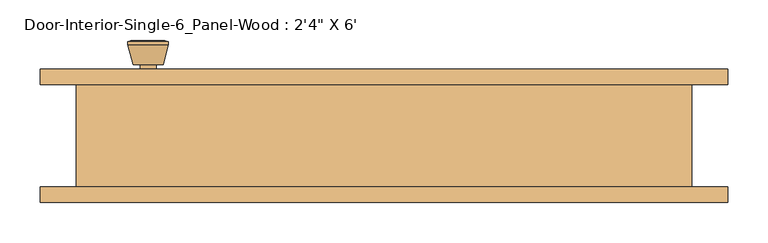
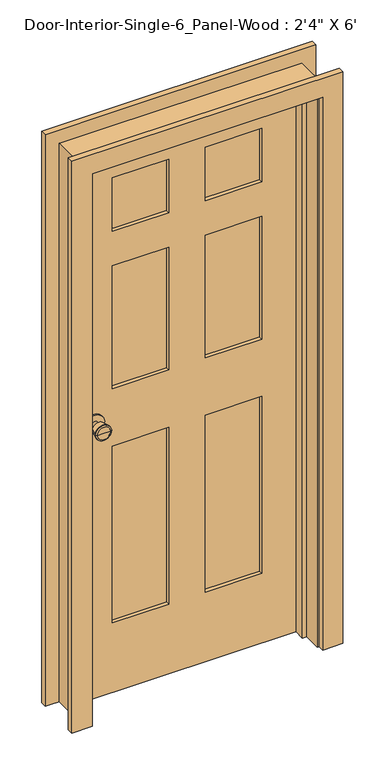
"""IFC4 building model written with IfcOpenShell, lengths in millimetres: door geometry."""

from ifc_helpers import new_model, si_unit, point, frame, frame_2d, origin, place, context, project, spatial, polyline, circle_curve, trimmed, segment, composite_curve, outline, extrude, faceted_brep, source, transform, mapped, element, save
from ifc_brep_helpers import plane_surface, cylinder_surface, revolved_surface, advanced_brep


def door_56a52d02(model_context):
    return source(origin(), model_context, "Body", "SolidModel", [
        advanced_brep(
        [(-292.1, 19.4, 914.4), (-282.1, 19.4, 914.4), (-302.1, 19.4, 914.4), (-271.6241324, -29.6, 914.4), (-292.1, -29.6, 914.4), (-312.5758676, -29.6, 914.4), (-267.1, -27.7721319, 914.4), (-317.1, -27.7721319, 914.4), (-267.1, -24.3084537, 914.4), (-317.1, -24.3084537, 914.4), (-273.463764, 0.4, 914.4), (-310.736236, 0.4, 914.4), (-282.1, 0.4, 914.4), (-302.1, 0.4, 914.4)],
        [
            (0, 1),
            (1, 2, circle_curve(frame((-292.1, 19.4, 914.4), z_axis=(0.0, 1.0, 0.0), x_axis=(-1.0, 0.0, 0.0)), 10.0)),
            (2, 0),
            (2, 1, circle_curve(frame((-292.1, 19.4, 914.4), z_axis=(0.0, 1.0, 0.0), x_axis=(-1.0, 0.0, 0.0)), 10.0)),
            (3, 4),
            (4, 5),
            (5, 3, circle_curve(frame((-292.1, -29.6, 914.4), z_axis=(0.0, -1.0, 0.0), x_axis=(-1.0, 0.0, 0.0)), 20.4758676)),
            (3, 5, circle_curve(frame((-292.1, -29.6, 914.4), z_axis=(0.0, -1.0, 0.0), x_axis=(-1.0, 0.0, 0.0)), 20.4758676)),
            (6, 3),
            (5, 7),
            (7, 6, circle_curve(frame((-292.1, -27.7721319, 914.4), z_axis=(0.0, -1.0, 0.0), x_axis=(-1.0, 0.0, 0.0)), 25.0)),
            (6, 7, circle_curve(frame((-292.1, -27.7721319, 914.4), z_axis=(0.0, -1.0, 0.0), x_axis=(-1.0, 0.0, 0.0)), 25.0)),
            (8, 6),
            (7, 9),
            (9, 8, circle_curve(frame((-292.1, -24.3084537, 914.4), z_axis=(0.0, -1.0, 0.0), x_axis=(-1.0, 0.0, 0.0)), 25.0)),
            (8, 9, circle_curve(frame((-292.1, -24.3084537, 914.4), z_axis=(0.0, -1.0, 0.0), x_axis=(-1.0, 0.0, 0.0)), 25.0)),
            (10, 8),
            (9, 11),
            (11, 10, circle_curve(frame((-292.1, 0.4, 914.4), z_axis=(0.0, -1.0, 0.0), x_axis=(-1.0, 0.0, 0.0)), 18.636236)),
            (10, 11, circle_curve(frame((-292.1, 0.4, 914.4), z_axis=(0.0, -1.0, 0.0), x_axis=(-1.0, 0.0, 0.0)), 18.636236)),
            (12, 10),
            (11, 13),
            (13, 12, circle_curve(frame((-292.1, 0.4, 914.4), z_axis=(0.0, -1.0, 0.0), x_axis=(-1.0, 0.0, 0.0)), 10.0)),
            (12, 13, circle_curve(frame((-292.1, 0.4, 914.4), z_axis=(0.0, -1.0, 0.0), x_axis=(-1.0, 0.0, 0.0)), 10.0)),
            (1, 12),
            (13, 2),
        ],
        [
            plane_surface(frame((-292.1, 19.4, 914.4), z_axis=(0.0, 1.0, 0.0), x_axis=(-1.0, 0.0, 0.0))),
            plane_surface(frame((-292.1, -29.6, 914.4), z_axis=(0.0, -1.0, 0.0), x_axis=(-1.0, 0.0, 0.0))),
            revolved_surface(polyline([(-312.5758676, -29.6, 914.4), (-317.1, -27.7721319, 914.4)]), (-292.1, 19.4, 914.4), (0.0, 1.0, 0.0)),
            cylinder_surface(frame((-292.1, 19.4, 914.4), z_axis=(0.0, 1.0, 0.0), x_axis=(-1.0, 0.0, 0.0)), 25.0),
            revolved_surface(polyline([(-317.1, -24.3084537, 914.4), (-310.736236, 0.4, 914.4)]), (-292.1, 19.4, 914.4), (0.0, 1.0, 0.0)),
            plane_surface(frame((-292.1, 0.4, 914.4), z_axis=(0.0, 1.0, 0.0), x_axis=(-1.0, 0.0, 0.0))),
            cylinder_surface(frame((-292.1, 19.4, 914.4), z_axis=(0.0, 1.0, 0.0), x_axis=(-1.0, 0.0, 0.0)), 10.0),
        ],
        [
            (0, [[1, 2, 3]]),
            (0, [[-3, 4, -1]]),
            (1, [[5, 6, 7]]),
            (1, [[-6, -5, 8]]),
            (2, [[9, -7, 10, 11]]),
            (2, [[-10, -8, -9, 12]]),
            (3, [[13, -11, 14, 15]]),
            (3, [[-14, -12, -13, 16]]),
            (4, [[17, -15, 18, 19]]),
            (4, [[-18, -16, -17, 20]]),
            (5, [[21, -19, 22, 23]]),
            (5, [[-22, -20, -21, 24]]),
            (6, [[25, -23, 26, -2]]),
            (6, [[-26, -24, -25, -4]]),
        ],
    ),
        extrude(outline(composite_curve([segment(trimmed(circle_curve(frame_2d((914.4, -292.1)), 30.0), [point((914.4, -322.1))], [point((914.4, -262.1))], False, "CARTESIAN"), True, "CONTINUOUS"), segment(trimmed(circle_curve(frame_2d((914.4, -292.1)), 30.0), [point((914.4, -262.1))], [point((914.4, -322.1))], False, "CARTESIAN"), True, "CONTINUOUS")], self_intersect=False)), frame((0.0, 19.4, 0.0), z_axis=(0.0, 1.0, 0.0), x_axis=(0.0, 0.0, 1.0)), (0.0, 0.0, 1.0), 6.0),
        advanced_brep(
        [(-292.1, 66.325, 914.4), (-302.1, 66.325, 914.4), (-282.1, 66.325, 914.4), (-271.6241324, 115.325, 914.4), (-312.5758676, 115.325, 914.4), (-292.1, 115.325, 914.4), (-267.1, 113.4971319, 914.4), (-317.1, 113.4971319, 914.4), (-267.1, 110.0334537, 914.4), (-317.1, 110.0334537, 914.4), (-273.463764, 85.325, 914.4), (-310.736236, 85.325, 914.4), (-282.1, 85.325, 914.4), (-302.1, 85.325, 914.4)],
        [
            (0, 1),
            (1, 2, circle_curve(frame((-292.1, 66.325, 914.4), z_axis=(0.0, -1.0, 0.0), x_axis=(-1.0, 0.0, 0.0)), 10.0)),
            (2, 0),
            (2, 1, circle_curve(frame((-292.1, 66.325, 914.4), z_axis=(0.0, -1.0, 0.0), x_axis=(-1.0, 0.0, 0.0)), 10.0)),
            (3, 4, circle_curve(frame((-292.1, 115.325, 914.4), z_axis=(0.0, 1.0, 0.0), x_axis=(-1.0, 0.0, 0.0)), 20.4758676)),
            (4, 5),
            (5, 3),
            (4, 3, circle_curve(frame((-292.1, 115.325, 914.4), z_axis=(0.0, 1.0, 0.0), x_axis=(-1.0, 0.0, 0.0)), 20.4758676)),
            (6, 7, circle_curve(frame((-292.1, 113.4971319, 914.4), z_axis=(0.0, 1.0, 0.0), x_axis=(-1.0, 0.0, 0.0)), 25.0)),
            (7, 4),
            (3, 6),
            (7, 6, circle_curve(frame((-292.1, 113.4971319, 914.4), z_axis=(0.0, 1.0, 0.0), x_axis=(-1.0, 0.0, 0.0)), 25.0)),
            (8, 9, circle_curve(frame((-292.1, 110.0334537, 914.4), z_axis=(0.0, 1.0, 0.0), x_axis=(-1.0, 0.0, 0.0)), 25.0)),
            (9, 7),
            (6, 8),
            (9, 8, circle_curve(frame((-292.1, 110.0334537, 914.4), z_axis=(0.0, 1.0, 0.0), x_axis=(-1.0, 0.0, 0.0)), 25.0)),
            (10, 11, circle_curve(frame((-292.1, 85.325, 914.4), z_axis=(0.0, 1.0, 0.0), x_axis=(-1.0, 0.0, 0.0)), 18.636236)),
            (11, 9),
            (8, 10),
            (11, 10, circle_curve(frame((-292.1, 85.325, 914.4), z_axis=(0.0, 1.0, 0.0), x_axis=(-1.0, 0.0, 0.0)), 18.636236)),
            (12, 13, circle_curve(frame((-292.1, 85.325, 914.4), z_axis=(0.0, 1.0, 0.0), x_axis=(-1.0, 0.0, 0.0)), 10.0)),
            (13, 11),
            (10, 12),
            (13, 12, circle_curve(frame((-292.1, 85.325, 914.4), z_axis=(0.0, 1.0, 0.0), x_axis=(-1.0, 0.0, 0.0)), 10.0)),
            (1, 13),
            (12, 2),
        ],
        [
            plane_surface(frame((-292.1, 66.325, 914.4), z_axis=(0.0, -1.0, 0.0), x_axis=(-1.0, 0.0, 0.0))),
            plane_surface(frame((-292.1, 115.325, 914.4), z_axis=(0.0, 1.0, 0.0), x_axis=(-1.0, 0.0, 0.0))),
            revolved_surface(polyline([(-312.5758676, 115.325, 914.4), (-317.1, 113.4971319, 914.4)]), (-292.1, 66.325, 914.4), (0.0, -1.0, 0.0)),
            cylinder_surface(frame((-292.1, 66.325, 914.4), z_axis=(0.0, -1.0, 0.0), x_axis=(-1.0, 0.0, 0.0)), 25.0),
            revolved_surface(polyline([(-317.1, 110.0334537, 914.4), (-310.736236, 85.325, 914.4)]), (-292.1, 66.325, 914.4), (0.0, -1.0, 0.0)),
            plane_surface(frame((-292.1, 85.325, 914.4), z_axis=(0.0, -1.0, 0.0), x_axis=(-1.0, 0.0, 0.0))),
            cylinder_surface(frame((-292.1, 66.325, 914.4), z_axis=(0.0, -1.0, 0.0), x_axis=(-1.0, 0.0, 0.0)), 10.0),
        ],
        [
            (0, [[1, 2, 3]]),
            (0, [[-3, 4, -1]]),
            (1, [[5, 6, 7]]),
            (1, [[8, -7, -6]]),
            (2, [[9, 10, -5, 11]]),
            (2, [[12, -11, -8, -10]]),
            (3, [[13, 14, -9, 15]]),
            (3, [[16, -15, -12, -14]]),
            (4, [[17, 18, -13, 19]]),
            (4, [[20, -19, -16, -18]]),
            (5, [[21, 22, -17, 23]]),
            (5, [[24, -23, -20, -22]]),
            (6, [[-2, 25, -21, 26]]),
            (6, [[-4, -26, -24, -25]]),
        ],
    ),
        extrude(outline(composite_curve([segment(trimmed(circle_curve(frame_2d((914.4, -292.1)), 30.0), [point((914.4, -322.1))], [point((914.4, -262.1))], False, "CARTESIAN"), True, "CONTINUOUS"), segment(trimmed(circle_curve(frame_2d((914.4, -292.1)), 30.0), [point((914.4, -262.1))], [point((914.4, -322.1))], False, "CARTESIAN"), True, "CONTINUOUS")], self_intersect=False)), frame((0.0, 60.325, 0.0), z_axis=(0.0, 1.0, 0.0), x_axis=(0.0, 0.0, 1.0)), (0.0, 0.0, 1.0), 6.0),
        faceted_brep([(381.0, 60.325, 0.0), (381.0, -66.675, 0.0), (355.6, -66.675, 0.0), (355.6, -9.525, 0.0), (342.9, -9.525, 0.0), (342.9, 25.4, 0.0), (355.6, 25.4, 0.0), (355.6, 60.325, 0.0), (381.0, 60.325, 1854.2), (381.0, -66.675, 1854.2), (-381.0, -66.675, 1854.2), (-381.0, -66.675, 0.0), (-355.6, -66.675, 0.0), (-355.6, -66.675, 1828.8), (355.6, -66.675, 1828.8), (355.6, -9.525, 1828.8), (-355.6, -9.525, 1828.8), (-355.6, -9.525, 0.0), (-342.9, -9.525, 0.0), (-342.9, -9.525, 1816.1), (342.9, -9.525, 1816.1), (342.9, 25.4, 1816.1), (-342.9, 25.4, 1816.1), (-342.9, 25.4, 0.0), (-355.6, 25.4, 0.0), (-355.6, 25.4, 1828.8), (355.6, 25.4, 1828.8), (355.6, 60.325, 1828.8), (-355.6, 60.325, 1828.8), (-355.6, 60.325, 0.0), (-381.0, 60.325, 0.0), (-381.0, 60.325, 1854.2)], [[[0, 1, 2, 3, 4, 5, 6, 7]], [[1, 0, 8, 9]], [[2, 1, 9, 10, 11, 12, 13, 14]], [[3, 2, 14, 15]], [[4, 3, 15, 16, 17, 18, 19, 20]], [[5, 4, 20, 21]], [[6, 5, 21, 22, 23, 24, 25, 26]], [[7, 6, 26, 27]], [[0, 7, 27, 28, 29, 30, 31, 8]], [[9, 8, 31, 10]], [[15, 14, 13, 16]], [[21, 20, 19, 22]], [[27, 26, 25, 28]], [[30, 29, 24, 23, 18, 17, 12, 11]], [[10, 31, 30, 11]], [[16, 13, 12, 17]], [[22, 19, 18, 23]], [[28, 25, 24, 29]]]),
        extrude(outline(polyline([(1828.8, -355.6), (0.0, -355.6), (0.0, 355.6), (1828.8, 355.6), (1828.8, -355.6)]), holes=[polyline([(1709.7375, 57.15), (1709.7375, 234.95), (1531.9375, 234.95), (1531.9375, 57.15), (1709.7375, 57.15)]), polyline([(1417.6375, 234.95), (1009.65, 234.95), (1009.65, 57.15), (1417.6375, 57.15), (1417.6375, 234.95)]), polyline([(1009.65, -57.15), (1009.65, -234.95), (1417.6375, -234.95), (1417.6375, -57.15), (1009.65, -57.15)]), polyline([(1531.9375, -234.95), (1709.7375, -234.95), (1709.7375, -57.15), (1531.9375, -57.15), (1531.9375, -234.95)]), polyline([(819.15, 57.15), (819.15, 234.95), (231.775, 234.95), (231.775, 57.15), (819.15, 57.15)]), polyline([(231.775, -57.15), (231.775, -234.95), (819.15, -234.95), (819.15, -57.15), (231.775, -57.15)])]), frame((0.0, 25.4, 0.0), z_axis=(0.0, 1.0, 0.0), x_axis=(0.0, 0.0, 1.0)), (0.0, 0.0, 1.0), 34.925),
        extrude(outline(polyline([(234.95, 37.0416667), (57.15, 37.0416667), (57.15, 48.6833333), (234.95, 48.6833333), (234.95, 37.0416667)])), frame((0.0, 0.0, 1531.9375), z_axis=(0.0, 0.0, 1.0), x_axis=(1.0, 0.0, 0.0)), (0.0, 0.0, 1.0), 177.8),
        extrude(outline(polyline([(234.95, 37.0416667), (57.15, 37.0416667), (57.15, 48.6833333), (234.95, 48.6833333), (234.95, 37.0416667)])), frame((0.0, 0.0, 1009.65), z_axis=(0.0, 0.0, 1.0), x_axis=(1.0, 0.0, 0.0)), (0.0, 0.0, 1.0), 407.9875),
        extrude(outline(polyline([(-57.15, 37.0416667), (-234.95, 37.0416667), (-234.95, 48.6833333), (-57.15, 48.6833333), (-57.15, 37.0416667)])), frame((0.0, 0.0, 1009.65), z_axis=(0.0, 0.0, 1.0), x_axis=(1.0, 0.0, 0.0)), (0.0, 0.0, 1.0), 407.9875),
        extrude(outline(polyline([(-57.15, 37.0416667), (-234.95, 37.0416667), (-234.95, 48.6833333), (-57.15, 48.6833333), (-57.15, 37.0416667)])), frame((0.0, 0.0, 1531.9375), z_axis=(0.0, 0.0, 1.0), x_axis=(1.0, 0.0, 0.0)), (0.0, 0.0, 1.0), 177.8),
        extrude(outline(polyline([(234.95, 37.0416667), (57.15, 37.0416667), (57.15, 48.6833333), (234.95, 48.6833333), (234.95, 37.0416667)])), frame((0.0, 0.0, 231.775), z_axis=(0.0, 0.0, 1.0), x_axis=(1.0, 0.0, 0.0)), (0.0, 0.0, 1.0), 587.375),
        extrude(outline(polyline([(-57.15, 37.0416667), (-234.95, 37.0416667), (-234.95, 48.6833333), (-57.15, 48.6833333), (-57.15, 37.0416667)])), frame((0.0, 0.0, 231.775), z_axis=(0.0, 0.0, 1.0), x_axis=(1.0, 0.0, 0.0)), (0.0, 0.0, 1.0), 587.375),
        extrude(outline(polyline([(0.0, 361.95), (0.0, 425.45), (1898.65, 425.45), (1898.65, -425.45), (0.0, -425.45), (0.0, -361.95), (1835.15, -361.95), (1835.15, 361.95), (0.0, 361.95)])), frame((0.0, 60.325, 0.0), z_axis=(0.0, 1.0, 0.0), x_axis=(0.0, 0.0, 1.0)), (0.0, 0.0, 1.0), 19.05),
        extrude(outline(polyline([(0.0, 361.95), (0.0, 425.45), (1898.65, 425.45), (1898.65, -425.45), (0.0, -425.45), (0.0, -361.95), (1835.15, -361.95), (1835.15, 361.95), (0.0, 361.95)])), frame((0.0, -85.725, 0.0), z_axis=(0.0, 1.0, 0.0), x_axis=(0.0, 0.0, 1.0)), (0.0, 0.0, 1.0), 19.05),
    ])


if __name__ == "__main__":
    model = new_model("IFC4")
    model_context = context("Model", 3, world=origin())
    ifc_project = project(units=[si_unit("LENGTHUNIT", "METRE", prefix="MILLI")], contexts=[model_context])
    site = spatial("IfcSite", under=ifc_project)
    building = spatial("IfcBuilding", under=site)
    placement = place(None, origin())
    door_shape = door_56a52d02(model_context)
    element("IfcDoor", 1, ObjectType="Door-Interior-Single-6_Panel-Wood : 2'4\" X 6'", at=placement, inside=building, context=model_context, shape_type="MappedRepresentation", body=[
        mapped(door_shape, transform((0.0, 0.0, 0.0), x_axis=(1.0, 0.0, 0.0), y_axis=(0.0, 1.0, 0.0), z_axis=(0.0, 0.0, 1.0))),
    ])
    save(model, "model.ifc")

# Revit data of these elements
# Type "Door-Interior-Single-6_Panel-Wood : 2'4\" X 6'"
#   Type Mark = "15"
#   Assembly Code = "C1020300"
#   Analytic Construction = "Wooden"
#   Top Rail = 0' - 4 11/16"
#   Top Panel = 0' - 7"
#   Thickness = 0' - 1 3/8"
#   Thermal Resistance (R) = 2.5876 (h·ft²·°F)/BTU
#   Swing Angle [instance default] = 90.00°
#   Stiles = 0' - 4 3/4"
#   Rough Width = 2' - 6"
#   Rough Height = 6' - 1"
#   Mullion = 0' - 4 1/2"
#   Lock Rail = 0' - 7 1/2"
#   Intermediate Rail = 0' - 4 1/2"
#   Height = 6' - 0"
#   Width = 2' - 4"
#   Heat Transfer Coefficient (U) = 0.3865 BTU/(h·ft²·°F)
#   Bottom Rail = 0' - 9 1/8"
#   Trim Material = Cherry
#   Panel Material = Cherry
#   Frame Material = Cherry
#   Door Handle Material = Aluminum
#   Visual Light Transmittance = 0
#   Solar Heat Gain Coefficient = 0
#   Wall Closure = (empty or 0)
#   Function = (empty or 0)
# Element 1 (IfcDoor, "Door-Interior-Single-6_Panel-Wood : 2'4\" X 6'")
#   Materials on its faces: "Cherry", "Aluminum"
# Materials
#   "Cherry": class "Wood", colour RGB 226 177 128, transparency 0, Description = "Prunus Serotina", Cost = 0
#   "Aluminum": class "Metal", colour RGB 247 247 247, transparency 0, Description = "Aluminum 6061", Cost = 0
